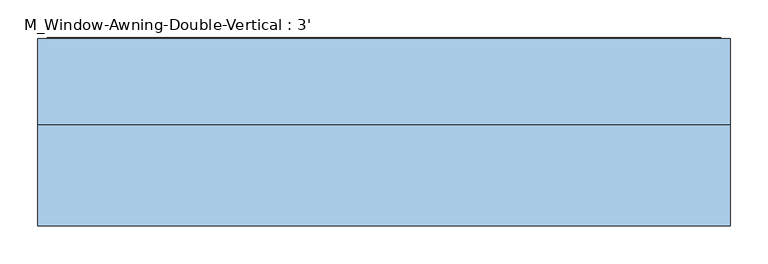
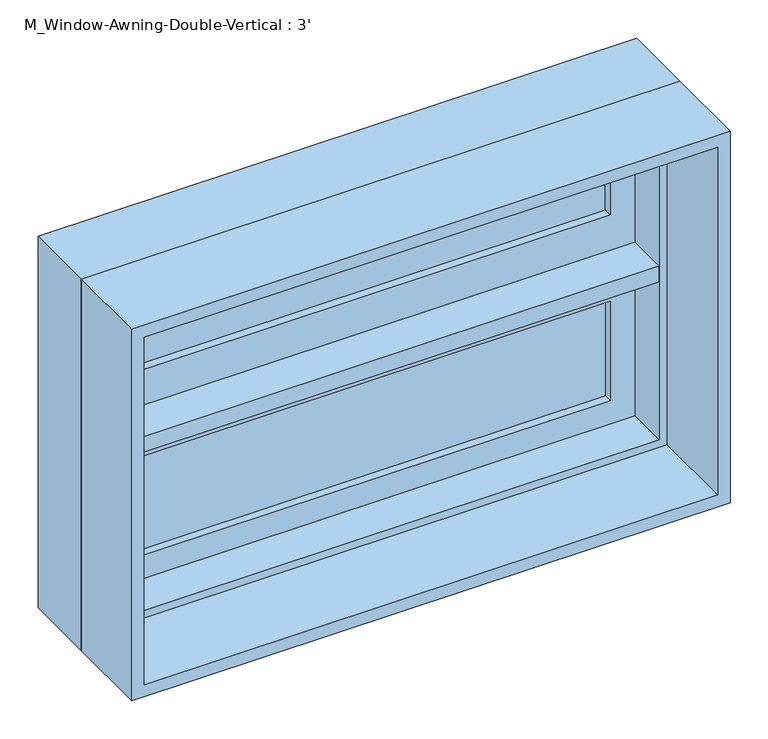
"""IFC4 building model written with IfcOpenShell, lengths in millimetres: window geometry, M_Window-Awning-Double-Vertical : 3'."""

from ifc_helpers import new_model, si_unit, frame, origin, place, context, project, spatial, polyline, outline, extrude, faceted_brep, source, transform, mapped, element, save


def m_window_awning_double_vertical_3_7e34f04a(model_context):
    return source(origin(), model_context, "Body", "SolidModel", [
        extrude(outline(polyline([(1500.0, -457.2), (900.0, -457.2), (900.0, 457.2), (1500.0, 457.2), (1500.0, -457.2)]), holes=[polyline([(1480.95, -438.15), (1480.95, 438.15), (919.05, 438.15), (919.05, -438.15), (1480.95, -438.15)])]), frame((0.0, -114.3, 0.0), z_axis=(0.0, 1.0, 0.0), x_axis=(0.0, 0.0, 1.0)), (0.0, 0.0, 1.0), 133.35),
        faceted_brep([(-457.2, 19.05, 1500.0), (-457.2, 133.35, 1500.0), (-457.2, 133.35, 900.0), (-457.2, 19.05, 900.0), (-444.5, 133.35, 1487.3), (-444.5, 82.55, 1487.3), (-444.5, 82.55, 912.7), (-444.5, 133.35, 912.7), (-425.45, 82.55, 1468.25), (-425.45, 19.05, 1468.25), (-425.45, 19.05, 931.75), (-425.45, 82.55, 931.75), (457.2, 133.35, 900.0), (457.2, 19.05, 900.0), (444.5, 82.55, 912.7), (444.5, 133.35, 912.7), (425.45, 19.05, 931.75), (425.45, 82.55, 931.75), (457.2, 133.35, 1500.0), (457.2, 19.05, 1500.0), (444.5, 82.55, 1487.3), (444.5, 133.35, 1487.3), (425.45, 19.05, 1468.25), (425.45, 82.55, 1468.25)], [[[0, 1, 2, 3]], [[4, 5, 6, 7]], [[8, 9, 10, 11]], [[3, 2, 12, 13]], [[7, 6, 14, 15]], [[11, 10, 16, 17]], [[13, 12, 18, 19]], [[15, 14, 20, 21]], [[17, 16, 22, 23]], [[3, 13, 19, 0], [9, 22, 16, 10]], [[19, 18, 1, 0]], [[1, 18, 12, 2], [7, 15, 21, 4]], [[21, 20, 5, 4]], [[5, 20, 14, 6], [11, 17, 23, 8]], [[23, 22, 9, 8]]]),
        extrude(outline(polyline([(1212.7, -444.5), (1212.7, 444.5), (1487.3, 444.5), (1487.3, -444.5), (1212.7, -444.5)]), holes=[polyline([(1430.15, -387.35), (1430.15, 387.35), (1269.85, 387.35), (1269.85, -387.35), (1430.15, -387.35)])]), frame((0.0, 82.55, 0.0), z_axis=(0.0, 1.0, 0.0), x_axis=(0.0, 0.0, 1.0)), (0.0, 0.0, 1.0), 44.45),
        extrude(outline(polyline([(387.35, 114.3), (387.35, 107.95), (-387.35, 107.95), (-387.35, 114.3), (387.35, 114.3)])), frame((0.0, 0.0, 1269.85), z_axis=(0.0, 0.0, 1.0), x_axis=(1.0, 0.0, 0.0)), (0.0, 0.0, 1.0), 160.3),
        extrude(outline(polyline([(387.35, 101.6), (387.35, 95.25), (-387.35, 95.25), (-387.35, 101.6), (387.35, 101.6)])), frame((0.0, 0.0, 1269.85), z_axis=(0.0, 0.0, 1.0), x_axis=(1.0, 0.0, 0.0)), (0.0, 0.0, 1.0), 160.3),
        extrude(outline(polyline([(387.35, 114.3), (387.35, 107.95), (-387.35, 107.95), (-387.35, 114.3), (387.35, 114.3)])), frame((0.0, 0.0, 969.85), z_axis=(0.0, 0.0, 1.0), x_axis=(1.0, 0.0, 0.0)), (0.0, 0.0, 1.0), 160.3),
        extrude(outline(polyline([(387.35, 101.6), (387.35, 95.25), (-387.35, 95.25), (-387.35, 101.6), (387.35, 101.6)])), frame((0.0, 0.0, 969.85), z_axis=(0.0, 0.0, 1.0), x_axis=(1.0, 0.0, 0.0)), (0.0, 0.0, 1.0), 160.3),
        extrude(outline(polyline([(-444.5, 82.55), (-444.5, 134.55), (444.5, 134.55), (444.5, 82.55), (425.45, 82.55), (425.45, 19.05), (-425.45, 19.05), (-425.45, 82.55), (-444.5, 82.55)])), frame((0.0, 0.0, 1187.3), z_axis=(0.0, 0.0, 1.0), x_axis=(1.0, 0.0, 0.0)), (0.0, 0.0, 1.0), 25.4),
        extrude(outline(polyline([(912.7, 444.5), (1187.3, 444.5), (1187.3, -444.5), (912.7, -444.5), (912.7, 444.5)]), holes=[polyline([(969.85, -387.35), (1130.15, -387.35), (1130.15, 387.35), (969.85, 387.35), (969.85, -387.35)])]), frame((0.0, 82.55, 0.0), z_axis=(0.0, 1.0, 0.0), x_axis=(0.0, 0.0, 1.0)), (0.0, 0.0, 1.0), 44.45),
    ])


if __name__ == "__main__":
    model = new_model("IFC4")
    model_context = context("Model", 3, world=origin())
    ifc_project = project(units=[si_unit("LENGTHUNIT", "METRE", prefix="MILLI")], contexts=[model_context])
    site = spatial("IfcSite", under=ifc_project)
    building = spatial("IfcBuilding", under=site)
    placement = place(None, origin())
    m_window_awning_double_vertical_3_shape = m_window_awning_double_vertical_3_7e34f04a(model_context)
    element("IfcWindow", 1, ObjectType="M_Window-Awning-Double-Vertical : 3'", at=placement, inside=building, context=model_context, shape_type="MappedRepresentation", body=[
        mapped(m_window_awning_double_vertical_3_shape, transform((0.0, 0.0, 0.0), x_axis=(1.0, 0.0, 0.0), y_axis=(0.0, 1.0, 0.0), z_axis=(0.0, 0.0, 1.0))),
    ])
    save(model, "model.ifc")

# Revit data of these elements
# Type "M_Window-Awning-Double-Vertical : 3'"
#   Type Mark = "22"
#   Fire Rating = "0.5h"
#   Assembly Code = "B2020100"
#   Analytic Construction = "Double glazing - domestic"
#   Window Inset [instance default] = 0' - 0"
#   Wall Thickness [instance default] = 0' - 5.90551"
#   Visual Light Transmittance = 0.81
#   Top Sash Height Ratio = 0.5
#   Top Sash Height = 0' - 11.81102"
#   Thermal Resistance (R) = 1.8146 (h·ft²·°F)/BTU
#   Solar Heat Gain Coefficient = 0.76
#   Rough Width = 3' - 0.59055"
#   Rough Height = 2' - 0.2126"
#   Interior Wall Closure [instance default] = 0' - 2.15551"
#   Height = 1' - 11.62205"
#   Heat Transfer Coefficient (U) = 0.5511 BTU/(h·ft²·°F)
#   Frame Extension [instance default] = 0' - 0 1/4"
#   Exterior Wall Closure [instance default] = 0' - 1 1/4"
#   Extension Jamb [instance default] = 0' - 2.15551"
#   Default Sill Height = 2' - 11.43307"
#   Width = 3' - 0"
#   Top Muntin Visibility = yes
#   Interior Trim Visibility [instance default] = yes
#   Exterior Trim Visibility [instance default] = yes
#   Extension Jamb Visibility [instance default] = yes
#   Bottom Muntin Visibility = yes
#   Muntin Pattern = M_Muntin Pattern_2x2 : M_Muntin Pattern_2x2
#   Interior Trim Material = Wood - Stained
#   Interior Trim = M_Trim-Window-Interior-Flat : Picture Frame
#   Interior Frame Material = Wood - Stained
#   Glass Panel Material = Glass
#   Exterior Trim Material = Clad - White
#   Exterior Trim = M_Trim-Window-Exterior-Flat : with Sill
#   Exterior Frame Material = Clad - White
#   Wall Closure = (empty or 0)
# Element 1 (IfcWindow, "M_Window-Awning-Double-Vertical : 3'")
#   Wall Thickness = 0' - 9"
#   Extension Jamb = 0' - 5 1/4"
#   Materials on its faces: "Wood - Stained", "Glass", "Clad - White"
# Materials
#   "Wood - Stained": class "Wood", colour RGB 224 178 126, transparency 0, Cost = 0
#   "Glass": class "Glass", colour RGB 0 128 192, transparency 0.75, Description = "Soda Lime Glass", Cost = 0
#   "Clad - White": class "Wood", colour RGB 242 242 238, transparency 0, Cost = 0
